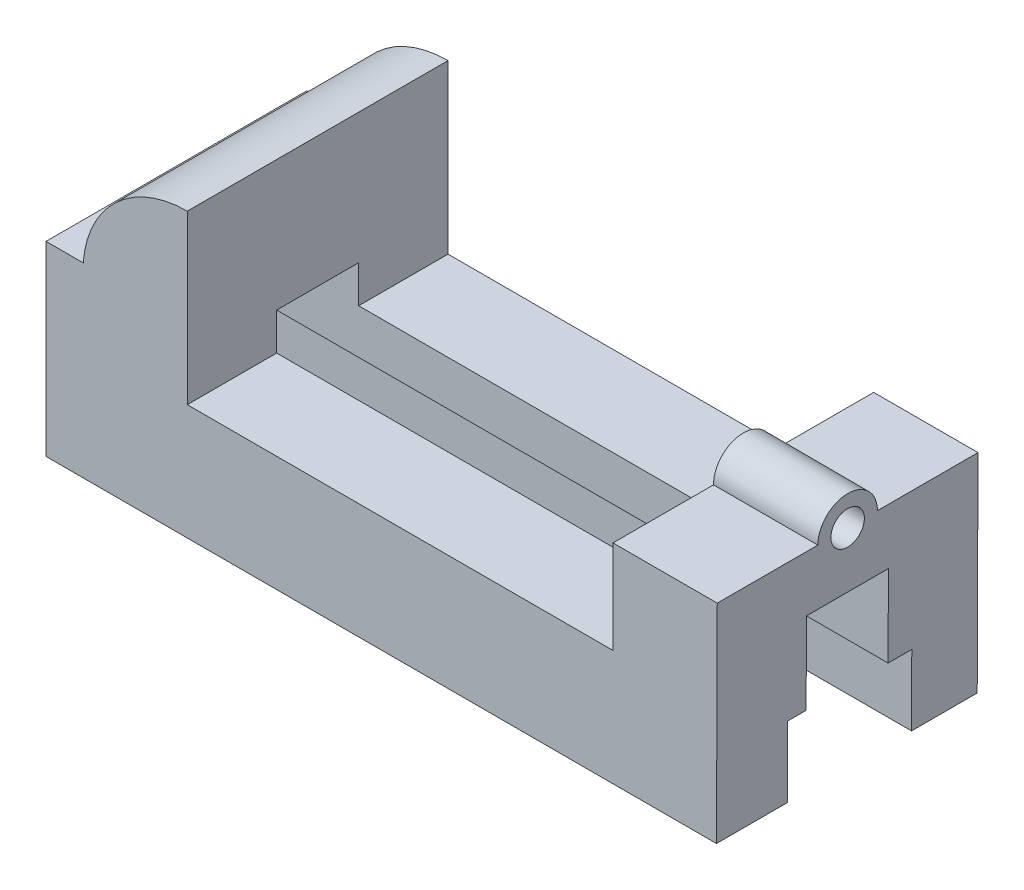
ISO-10303-21;
HEADER;
FILE_DESCRIPTION(('STEP AP214'),'2;1');
FILE_NAME('part.step','',(''),(''),'','','');
FILE_SCHEMA(('AUTOMOTIVE_DESIGN { 1 0 10303 214 1 1 1 1 }'));
ENDSEC;
DATA;
#1=APPLICATION_CONTEXT('core data for automotive mechanical design processes');
#2=APPLICATION_PROTOCOL_DEFINITION('international standard','automotive_design',2000,#1);
#3=PRODUCT_CONTEXT('',#1,'mechanical');
#4=PRODUCT('Part','Part','',(#3));
#5=PRODUCT_RELATED_PRODUCT_CATEGORY('part','',(#4));
#6=PRODUCT_DEFINITION_FORMATION('','',#4);
#7=PRODUCT_DEFINITION_CONTEXT('part definition',#1,'design');
#8=PRODUCT_DEFINITION('design','',#6,#7);
#9=PRODUCT_DEFINITION_SHAPE('','',#8);
#10=(LENGTH_UNIT() NAMED_UNIT(*) SI_UNIT(.MILLI.,.METRE.));
#11=(NAMED_UNIT(*) PLANE_ANGLE_UNIT() SI_UNIT($,.RADIAN.));
#12=(NAMED_UNIT(*) SI_UNIT($,.STERADIAN.) SOLID_ANGLE_UNIT());
#13=UNCERTAINTY_MEASURE_WITH_UNIT(LENGTH_MEASURE(1.E-05),#10,'distance_accuracy_value','');
#14=(GEOMETRIC_REPRESENTATION_CONTEXT(3) GLOBAL_UNCERTAINTY_ASSIGNED_CONTEXT((#13)) GLOBAL_UNIT_ASSIGNED_CONTEXT((#10,
#11,#12)) REPRESENTATION_CONTEXT('',''));
#15=CARTESIAN_POINT('',(0.,0.,0.));
#16=DIRECTION('',(0.,0.,1.));
#17=DIRECTION('',(1.,0.,0.));
#18=AXIS2_PLACEMENT_3D('',#15,#16,#17);
#19=CARTESIAN_POINT('',(152.209078325316,30.9996096973352,-70.));
#20=DIRECTION('',(0.,1.,0.));
#21=DIRECTION('',(-1.,0.,0.));
#22=AXIS2_PLACEMENT_3D('',#19,#20,#21);
#23=PLANE('',#22);
#24=DIRECTION('',(-1.,0.,0.));
#25=VECTOR('',#24,1.);
#26=CARTESIAN_POINT('',(152.209078325316,30.9996096973352,-46.));
#27=LINE('',#26,#25);
#28=CARTESIAN_POINT('',(152.209078325316,30.9996096973352,-46.));
#29=VERTEX_POINT('',#28);
#30=CARTESIAN_POINT('',(37.9284521346423,30.9996096973352,-46.));
#31=VERTEX_POINT('',#30);
#32=EDGE_CURVE('E288',#29,#31,#27,.T.);
#33=ORIENTED_EDGE('',*,*,#32,.F.);
#34=DIRECTION('',(0.,0.,1.));
#35=VECTOR('',#34,1.);
#36=CARTESIAN_POINT('',(152.209078325316,30.9996096973352,-70.));
#37=LINE('',#36,#35);
#38=CARTESIAN_POINT('',(152.209078325316,30.9996096973352,-70.));
#39=VERTEX_POINT('',#38);
#40=EDGE_CURVE('E364',#39,#29,#37,.T.);
#41=ORIENTED_EDGE('',*,*,#40,.F.);
#42=DIRECTION('',(-1.,0.,0.));
#43=VECTOR('',#42,1.);
#44=CARTESIAN_POINT('',(152.209078325316,30.9996096973352,-70.));
#45=LINE('',#44,#43);
#46=CARTESIAN_POINT('',(37.9284521346423,30.9996096973352,-70.));
#47=VERTEX_POINT('',#46);
#48=EDGE_CURVE('E324',#39,#47,#45,.T.);
#49=ORIENTED_EDGE('',*,*,#48,.T.);
#50=DIRECTION('',(0.,0.,1.));
#51=VECTOR('',#50,1.);
#52=CARTESIAN_POINT('',(37.9284521346423,30.9996096973352,-70.));
#53=LINE('',#52,#51);
#54=EDGE_CURVE('E363',#47,#31,#53,.T.);
#55=ORIENTED_EDGE('',*,*,#54,.T.);
#56=EDGE_LOOP('',(#33,#41,#49,#55));
#57=FACE_BOUND('',#56,.T.);
#58=ADVANCED_FACE('F39',(#57),#23,.T.);
#59=CARTESIAN_POINT('',(0.,0.,-70.));
#60=DIRECTION('',(0.,-1.,0.));
#61=DIRECTION('',(0.,0.,-1.));
#62=AXIS2_PLACEMENT_3D('',#59,#60,#61);
#63=PLANE('',#62);
#64=DIRECTION('',(1.,0.,0.));
#65=VECTOR('',#64,1.);
#66=CARTESIAN_POINT('',(0.,0.,-52.3591971480599));
#67=LINE('',#66,#65);
#68=CARTESIAN_POINT('',(0.,0.,-52.3591971480599));
#69=VERTEX_POINT('',#68);
#70=CARTESIAN_POINT('',(180.,0.,-52.3591971480599));
#71=VERTEX_POINT('',#70);
#72=EDGE_CURVE('E199',#69,#71,#67,.T.);
#73=ORIENTED_EDGE('',*,*,#72,.F.);
#74=DIRECTION('',(0.,0.,1.));
#75=VECTOR('',#74,1.);
#76=CARTESIAN_POINT('',(0.,0.,-70.));
#77=LINE('',#76,#75);
#78=CARTESIAN_POINT('',(0.,0.,-70.));
#79=VERTEX_POINT('',#78);
#80=EDGE_CURVE('E216',#79,#69,#77,.T.);
#81=ORIENTED_EDGE('',*,*,#80,.F.);
#82=DIRECTION('',(1.,0.,0.));
#83=VECTOR('',#82,1.);
#84=CARTESIAN_POINT('',(0.,0.,-70.));
#85=LINE('',#84,#83);
#86=CARTESIAN_POINT('',(180.,0.,-70.));
#87=VERTEX_POINT('',#86);
#88=EDGE_CURVE('E315',#79,#87,#85,.T.);
#89=ORIENTED_EDGE('',*,*,#88,.T.);
#90=DIRECTION('',(0.,0.,1.));
#91=VECTOR('',#90,1.);
#92=CARTESIAN_POINT('',(180.,0.,-70.));
#93=LINE('',#92,#91);
#94=EDGE_CURVE('E223',#87,#71,#93,.T.);
#95=ORIENTED_EDGE('',*,*,#94,.T.);
#96=EDGE_LOOP('',(#73,#81,#89,#95));
#97=FACE_BOUND('',#96,.T.);
#98=ADVANCED_FACE('F461',(#97),#63,.T.);
#99=CARTESIAN_POINT('',(180.209078325316,55.9996096973353,-70.));
#100=DIRECTION('',(0.,1.,0.));
#101=DIRECTION('',(0.,0.,1.));
#102=AXIS2_PLACEMENT_3D('',#99,#100,#101);
#103=PLANE('',#102);
#104=CARTESIAN_POINT('',(180.209078325316,55.9996096973353,-35.));
#105=DIRECTION('',(0.,1.,0.));
#106=DIRECTION('',(1.,0.,0.));
#107=AXIS2_PLACEMENT_3D('',#104,#105,#106);
#108=ELLIPSE('',#107,2142.73765261709,8.);
#109=CARTESIAN_POINT('',(180.209078325316,55.9996096973353,-43.));
#110=VERTEX_POINT('',#109);
#111=CARTESIAN_POINT('',(152.209078325316,55.9996096973353,-42.9993169435566));
#112=VERTEX_POINT('',#111);
#113=EDGE_CURVE('E307',#110,#112,#108,.T.);
#114=ORIENTED_EDGE('',*,*,#113,.F.);
#115=DIRECTION('',(0.,0.,1.));
#116=VECTOR('',#115,1.);
#117=CARTESIAN_POINT('',(180.209078325316,55.9996096973353,-70.));
#118=LINE('',#117,#116);
#119=CARTESIAN_POINT('',(180.209078325316,55.9996096973353,-70.));
#120=VERTEX_POINT('',#119);
#121=EDGE_CURVE('E375',#120,#110,#118,.T.);
#122=ORIENTED_EDGE('',*,*,#121,.F.);
#123=DIRECTION('',(-1.,0.,0.));
#124=VECTOR('',#123,1.);
#125=CARTESIAN_POINT('',(180.209078325316,55.9996096973353,-70.));
#126=LINE('',#125,#124);
#127=CARTESIAN_POINT('',(152.209078325316,55.9996096973353,-70.));
#128=VERTEX_POINT('',#127);
#129=EDGE_CURVE('E317',#120,#128,#126,.T.);
#130=ORIENTED_EDGE('',*,*,#129,.T.);
#131=DIRECTION('',(0.,0.,1.));
#132=VECTOR('',#131,1.);
#133=CARTESIAN_POINT('',(152.209078325316,55.9996096973353,-70.));
#134=LINE('',#133,#132);
#135=EDGE_CURVE('E369',#128,#112,#134,.T.);
#136=ORIENTED_EDGE('',*,*,#135,.T.);
#137=EDGE_LOOP('',(#114,#122,#130,#136));
#138=FACE_BOUND('',#137,.T.);
#139=ADVANCED_FACE('F413',(#138),#103,.T.);
#140=CARTESIAN_POINT('',(0.,50.,-70.));
#141=DIRECTION('',(-1.,0.,0.));
#142=DIRECTION('',(0.,-1.,0.));
#143=AXIS2_PLACEMENT_3D('',#140,#141,#142);
#144=PLANE('',#143);
#145=DIRECTION('',(0.,-1.,0.));
#146=VECTOR('',#145,1.);
#147=CARTESIAN_POINT('',(0.,0.,-52.3591971480599));
#148=LINE('',#147,#146);
#149=CARTESIAN_POINT('',(0.,19.,-52.3591971480599));
#150=VERTEX_POINT('',#149);
#151=EDGE_CURVE('E271',#150,#69,#148,.T.);
#152=ORIENTED_EDGE('',*,*,#151,.F.);
#153=DIRECTION('',(0.,0.,-1.));
#154=VECTOR('',#153,1.);
#155=CARTESIAN_POINT('',(0.,19.,-52.3591971480599));
#156=LINE('',#155,#154);
#157=CARTESIAN_POINT('',(0.,19.,-46.));
#158=VERTEX_POINT('',#157);
#159=EDGE_CURVE('E423',#158,#150,#156,.T.);
#160=ORIENTED_EDGE('',*,*,#159,.F.);
#161=DIRECTION('',(0.,-1.,0.));
#162=VECTOR('',#161,1.);
#163=CARTESIAN_POINT('',(0.,19.,-46.));
#164=LINE('',#163,#162);
#165=CARTESIAN_POINT('',(0.,41.,-46.));
#166=VERTEX_POINT('',#165);
#167=EDGE_CURVE('E652',#166,#158,#164,.T.);
#168=ORIENTED_EDGE('',*,*,#167,.F.);
#169=DIRECTION('',(0.,0.,-1.));
#170=VECTOR('',#169,1.);
#171=CARTESIAN_POINT('',(0.,41.,-46.));
#172=LINE('',#171,#170);
#173=CARTESIAN_POINT('',(0.,41.,-24.));
#174=VERTEX_POINT('',#173);
#175=EDGE_CURVE('E433',#174,#166,#172,.T.);
#176=ORIENTED_EDGE('',*,*,#175,.F.);
#177=DIRECTION('',(0.,1.,0.));
#178=VECTOR('',#177,1.);
#179=CARTESIAN_POINT('',(0.,41.,-24.));
#180=LINE('',#179,#178);
#181=CARTESIAN_POINT('',(0.,19.,-24.));
#182=VERTEX_POINT('',#181);
#183=EDGE_CURVE('E657',#182,#174,#180,.T.);
#184=ORIENTED_EDGE('',*,*,#183,.F.);
#185=DIRECTION('',(0.,0.,-1.));
#186=VECTOR('',#185,1.);
#187=CARTESIAN_POINT('',(0.,19.,-24.));
#188=LINE('',#187,#186);
#189=CARTESIAN_POINT('',(0.,19.,-19.));
#190=VERTEX_POINT('',#189);
#191=EDGE_CURVE('E209',#190,#182,#188,.T.);
#192=ORIENTED_EDGE('',*,*,#191,.F.);
#193=DIRECTION('',(0.,1.,0.));
#194=VECTOR('',#193,1.);
#195=CARTESIAN_POINT('',(0.,19.,-19.));
#196=LINE('',#195,#194);
#197=CARTESIAN_POINT('',(0.,0.,-19.));
#198=VERTEX_POINT('',#197);
#199=EDGE_CURVE('E191',#198,#190,#196,.T.);
#200=ORIENTED_EDGE('',*,*,#199,.F.);
#201=CARTESIAN_POINT('',(0.,0.,0.));
#202=VERTEX_POINT('',#201);
#203=EDGE_CURVE('E206',#198,#202,#77,.T.);
#204=ORIENTED_EDGE('',*,*,#203,.T.);
#205=DIRECTION('',(0.,-1.,0.));
#206=VECTOR('',#205,1.);
#207=CARTESIAN_POINT('',(0.,50.,0.));
#208=LINE('',#207,#206);
#209=CARTESIAN_POINT('',(0.,50.,0.));
#210=VERTEX_POINT('',#209);
#211=EDGE_CURVE('E334',#210,#202,#208,.T.);
#212=ORIENTED_EDGE('',*,*,#211,.F.);
#213=DIRECTION('',(0.,0.,1.));
#214=VECTOR('',#213,1.);
#215=CARTESIAN_POINT('',(0.,50.,-70.));
#216=LINE('',#215,#214);
#217=CARTESIAN_POINT('',(0.,50.,-70.));
#218=VERTEX_POINT('',#217);
#219=EDGE_CURVE('E203',#218,#210,#216,.T.);
#220=ORIENTED_EDGE('',*,*,#219,.F.);
#221=DIRECTION('',(0.,-1.,0.));
#222=VECTOR('',#221,1.);
#223=CARTESIAN_POINT('',(0.,50.,-70.));
#224=LINE('',#223,#222);
#225=EDGE_CURVE('E310',#218,#79,#224,.T.);
#226=ORIENTED_EDGE('',*,*,#225,.T.);
#227=ORIENTED_EDGE('',*,*,#80,.T.);
#228=EDGE_LOOP('',(#152,#160,#168,#176,#184,#192,#200,#204,#212,#220,#226,#227));
#229=FACE_BOUND('',#228,.T.);
#230=ADVANCED_FACE('F41',(#229),#144,.T.);
#231=CARTESIAN_POINT('',(10.,50.,-70.));
#232=DIRECTION('',(0.,1.,0.));
#233=DIRECTION('',(0.,0.,1.));
#234=AXIS2_PLACEMENT_3D('',#231,#232,#233);
#235=PLANE('',#234);
#236=DIRECTION('',(-1.,0.,0.));
#237=VECTOR('',#236,1.);
#238=CARTESIAN_POINT('',(10.,50.,0.));
#239=LINE('',#238,#237);
#240=CARTESIAN_POINT('',(10.,50.,0.));
#241=VERTEX_POINT('',#240);
#242=EDGE_CURVE('E311',#241,#210,#239,.T.);
#243=ORIENTED_EDGE('',*,*,#242,.F.);
#244=DIRECTION('',(0.,0.,1.));
#245=VECTOR('',#244,1.);
#246=CARTESIAN_POINT('',(10.,50.,-70.));
#247=LINE('',#246,#245);
#248=CARTESIAN_POINT('',(10.,50.,-70.));
#249=VERTEX_POINT('',#248);
#250=EDGE_CURVE('E360',#249,#241,#247,.T.);
#251=ORIENTED_EDGE('',*,*,#250,.F.);
#252=DIRECTION('',(-1.,0.,0.));
#253=VECTOR('',#252,1.);
#254=CARTESIAN_POINT('',(10.,50.,-70.));
#255=LINE('',#254,#253);
#256=EDGE_CURVE('E220',#249,#218,#255,.T.);
#257=ORIENTED_EDGE('',*,*,#256,.T.);
#258=ORIENTED_EDGE('',*,*,#219,.T.);
#259=EDGE_LOOP('',(#243,#251,#257,#258));
#260=FACE_BOUND('',#259,.T.);
#261=ADVANCED_FACE('F395',(#260),#235,.T.);
#262=CARTESIAN_POINT('',(37.9284521346423,47.9996096973352,-70.));
#263=DIRECTION('',(0.,0.,1.));
#264=DIRECTION('',(1.,0.,0.));
#265=AXIS2_PLACEMENT_3D('',#262,#263,#264);
#266=CYLINDRICAL_SURFACE('',#265,28.);
#267=CARTESIAN_POINT('',(37.9284521346423,47.9996096973352,0.));
#268=DIRECTION('',(0.,0.,1.));
#269=DIRECTION('',(1.,0.,0.));
#270=AXIS2_PLACEMENT_3D('',#267,#268,#269);
#271=CIRCLE('',#270,28.);
#272=CARTESIAN_POINT('',(37.9284521346423,75.9996096973352,0.));
#273=VERTEX_POINT('',#272);
#274=EDGE_CURVE('E351',#273,#241,#271,.T.);
#275=ORIENTED_EDGE('',*,*,#274,.F.);
#276=DIRECTION('',(0.,0.,1.));
#277=VECTOR('',#276,1.);
#278=CARTESIAN_POINT('',(37.9284521346423,75.9996096973352,-70.));
#279=LINE('',#278,#277);
#280=CARTESIAN_POINT('',(37.9284521346423,75.9996096973352,-70.));
#281=VERTEX_POINT('',#280);
#282=EDGE_CURVE('E359',#281,#273,#279,.T.);
#283=ORIENTED_EDGE('',*,*,#282,.F.);
#284=CARTESIAN_POINT('',(37.9284521346423,47.9996096973352,-70.));
#285=DIRECTION('',(0.,0.,1.));
#286=DIRECTION('',(1.,0.,0.));
#287=AXIS2_PLACEMENT_3D('',#284,#285,#286);
#288=CIRCLE('',#287,28.);
#289=EDGE_CURVE('E225',#281,#249,#288,.T.);
#290=ORIENTED_EDGE('',*,*,#289,.T.);
#291=ORIENTED_EDGE('',*,*,#250,.T.);
#292=EDGE_LOOP('',(#275,#283,#290,#291));
#293=FACE_BOUND('',#292,.T.);
#294=ADVANCED_FACE('F394',(#293),#266,.T.);
#295=CARTESIAN_POINT('',(37.9284521346423,30.9996096973352,-70.));
#296=DIRECTION('',(1.,0.,0.));
#297=DIRECTION('',(0.,0.,-1.));
#298=AXIS2_PLACEMENT_3D('',#295,#296,#297);
#299=PLANE('',#298);
#300=DIRECTION('',(0.,1.,0.));
#301=VECTOR('',#300,1.);
#302=CARTESIAN_POINT('',(37.9284521346423,30.9996096973352,-46.));
#303=LINE('',#302,#301);
#304=CARTESIAN_POINT('',(37.9284521346424,41.,-46.));
#305=VERTEX_POINT('',#304);
#306=EDGE_CURVE('E286',#31,#305,#303,.T.);
#307=ORIENTED_EDGE('',*,*,#306,.F.);
#308=ORIENTED_EDGE('',*,*,#54,.F.);
#309=DIRECTION('',(0.,1.,0.));
#310=VECTOR('',#309,1.);
#311=CARTESIAN_POINT('',(37.9284521346423,30.9996096973352,-70.));
#312=LINE('',#311,#310);
#313=EDGE_CURVE('E327',#47,#281,#312,.T.);
#314=ORIENTED_EDGE('',*,*,#313,.T.);
#315=ORIENTED_EDGE('',*,*,#282,.T.);
#316=DIRECTION('',(0.,1.,0.));
#317=VECTOR('',#316,1.);
#318=CARTESIAN_POINT('',(37.9284521346423,30.9996096973352,0.));
#319=LINE('',#318,#317);
#320=CARTESIAN_POINT('',(37.9284521346423,30.9996096973352,0.));
#321=VERTEX_POINT('',#320);
#322=EDGE_CURVE('E346',#321,#273,#319,.T.);
#323=ORIENTED_EDGE('',*,*,#322,.F.);
#324=CARTESIAN_POINT('',(37.9284521346423,30.9996096973352,-24.));
#325=VERTEX_POINT('',#324);
#326=EDGE_CURVE('E365',#325,#321,#53,.T.);
#327=ORIENTED_EDGE('',*,*,#326,.F.);
#328=DIRECTION('',(0.,-1.,0.));
#329=VECTOR('',#328,1.);
#330=CARTESIAN_POINT('',(37.9284521346423,30.9996096973352,-24.));
#331=LINE('',#330,#329);
#332=CARTESIAN_POINT('',(37.9284521346424,41.,-24.));
#333=VERTEX_POINT('',#332);
#334=EDGE_CURVE('E281',#333,#325,#331,.T.);
#335=ORIENTED_EDGE('',*,*,#334,.F.);
#336=DIRECTION('',(0.,0.,1.));
#337=VECTOR('',#336,1.);
#338=CARTESIAN_POINT('',(37.9284521346423,41.,-70.));
#339=LINE('',#338,#337);
#340=EDGE_CURVE('E283',#305,#333,#339,.T.);
#341=ORIENTED_EDGE('',*,*,#340,.F.);
#342=EDGE_LOOP('',(#307,#308,#314,#315,#323,#327,#335,#341));
#343=FACE_BOUND('',#342,.T.);
#344=ADVANCED_FACE('F396',(#343),#299,.T.);
#345=DIRECTION('',(1.,0.,0.));
#346=VECTOR('',#345,1.);
#347=CARTESIAN_POINT('',(152.209078325316,30.9996096973352,-24.));
#348=LINE('',#347,#346);
#349=CARTESIAN_POINT('',(152.209078325316,30.9996096973352,-24.));
#350=VERTEX_POINT('',#349);
#351=EDGE_CURVE('E53',#325,#350,#348,.T.);
#352=ORIENTED_EDGE('',*,*,#351,.F.);
#353=ORIENTED_EDGE('',*,*,#326,.T.);
#354=DIRECTION('',(-1.,0.,0.));
#355=VECTOR('',#354,1.);
#356=CARTESIAN_POINT('',(152.209078325316,30.9996096973352,0.));
#357=LINE('',#356,#355);
#358=CARTESIAN_POINT('',(152.209078325316,30.9996096973352,0.));
#359=VERTEX_POINT('',#358);
#360=EDGE_CURVE('E341',#359,#321,#357,.T.);
#361=ORIENTED_EDGE('',*,*,#360,.F.);
#362=EDGE_CURVE('E366',#350,#359,#37,.T.);
#363=ORIENTED_EDGE('',*,*,#362,.F.);
#364=EDGE_LOOP('',(#352,#353,#361,#363));
#365=FACE_BOUND('',#364,.T.);
#366=ADVANCED_FACE('F437',(#365),#23,.T.);
#367=CARTESIAN_POINT('',(152.209078325316,55.9996096973353,-70.));
#368=DIRECTION('',(-1.,0.,0.));
#369=DIRECTION('',(0.,0.,1.));
#370=AXIS2_PLACEMENT_3D('',#367,#368,#369);
#371=PLANE('',#370);
#372=DIRECTION('',(0.,-1.,0.));
#373=VECTOR('',#372,1.);
#374=CARTESIAN_POINT('',(152.209078325316,55.9996096973353,-46.));
#375=LINE('',#374,#373);
#376=CARTESIAN_POINT('',(152.209078325316,41.,-46.));
#377=VERTEX_POINT('',#376);
#378=EDGE_CURVE('E287',#377,#29,#375,.T.);
#379=ORIENTED_EDGE('',*,*,#378,.F.);
#380=DIRECTION('',(0.,0.,-1.));
#381=VECTOR('',#380,1.);
#382=CARTESIAN_POINT('',(152.209078325316,41.,-70.));
#383=LINE('',#382,#381);
#384=CARTESIAN_POINT('',(152.209078325316,41.,-24.));
#385=VERTEX_POINT('',#384);
#386=EDGE_CURVE('E252',#385,#377,#383,.T.);
#387=ORIENTED_EDGE('',*,*,#386,.F.);
#388=DIRECTION('',(0.,1.,0.));
#389=VECTOR('',#388,1.);
#390=CARTESIAN_POINT('',(152.209078325316,55.9996096973353,-24.));
#391=LINE('',#390,#389);
#392=EDGE_CURVE('E279',#350,#385,#391,.T.);
#393=ORIENTED_EDGE('',*,*,#392,.F.);
#394=ORIENTED_EDGE('',*,*,#362,.T.);
#395=DIRECTION('',(0.,-1.,0.));
#396=VECTOR('',#395,1.);
#397=CARTESIAN_POINT('',(152.209078325316,55.9996096973353,0.));
#398=LINE('',#397,#396);
#399=CARTESIAN_POINT('',(152.209078325316,55.9996096973353,0.));
#400=VERTEX_POINT('',#399);
#401=EDGE_CURVE('E345',#400,#359,#398,.T.);
#402=ORIENTED_EDGE('',*,*,#401,.F.);
#403=CARTESIAN_POINT('',(152.209078325316,55.9996096973353,-27.0006830564435));
#404=VERTEX_POINT('',#403);
#405=EDGE_CURVE('E371',#404,#400,#134,.T.);
#406=ORIENTED_EDGE('',*,*,#405,.F.);
#407=CARTESIAN_POINT('',(152.209078325316,56.1041495886038,-35.));
#408=DIRECTION('',(-1.,0.,0.));
#409=DIRECTION('',(0.,-1.,0.));
#410=AXIS2_PLACEMENT_3D('',#407,#408,#409);
#411=ELLIPSE('',#410,8.00005575791215,8.);
#412=EDGE_CURVE('E308',#112,#404,#411,.T.);
#413=ORIENTED_EDGE('',*,*,#412,.F.);
#414=ORIENTED_EDGE('',*,*,#135,.F.);
#415=DIRECTION('',(0.,-1.,0.));
#416=VECTOR('',#415,1.);
#417=CARTESIAN_POINT('',(152.209078325316,55.9996096973353,-70.));
#418=LINE('',#417,#416);
#419=EDGE_CURVE('E325',#128,#39,#418,.T.);
#420=ORIENTED_EDGE('',*,*,#419,.T.);
#421=ORIENTED_EDGE('',*,*,#40,.T.);
#422=EDGE_LOOP('',(#379,#387,#393,#394,#402,#406,#413,#414,#420,#421));
#423=FACE_BOUND('',#422,.T.);
#424=ADVANCED_FACE('F407',(#423),#371,.T.);
#425=CARTESIAN_POINT('',(180.209078325316,55.9996096973353,-27.));
#426=VERTEX_POINT('',#425);
#427=EDGE_CURVE('E305',#404,#426,#108,.T.);
#428=ORIENTED_EDGE('',*,*,#427,.F.);
#429=ORIENTED_EDGE('',*,*,#405,.T.);
#430=DIRECTION('',(-1.,0.,0.));
#431=VECTOR('',#430,1.);
#432=CARTESIAN_POINT('',(180.209078325316,55.9996096973353,0.));
#433=LINE('',#432,#431);
#434=CARTESIAN_POINT('',(180.209078325316,55.9996096973353,0.));
#435=VERTEX_POINT('',#434);
#436=EDGE_CURVE('E338',#435,#400,#433,.T.);
#437=ORIENTED_EDGE('',*,*,#436,.F.);
#438=EDGE_CURVE('E372',#426,#435,#118,.T.);
#439=ORIENTED_EDGE('',*,*,#438,.F.);
#440=EDGE_LOOP('',(#428,#429,#437,#439));
#441=FACE_BOUND('',#440,.T.);
#442=ADVANCED_FACE('F444',(#441),#103,.T.);
#443=CARTESIAN_POINT('',(180.,0.,-70.));
#444=DIRECTION('',(0.999993030309558,-0.00373354152349401,0.));
#445=DIRECTION('',(0.00373354152349401,0.999993030309558,0.));
#446=AXIS2_PLACEMENT_3D('',#443,#444,#445);
#447=PLANE('',#446);
#448=DIRECTION('',(0.00373354152349401,0.999993030309558,0.));
#449=VECTOR('',#448,1.);
#450=CARTESIAN_POINT('',(180.,0.,-52.3591971480599));
#451=LINE('',#450,#449);
#452=CARTESIAN_POINT('',(180.070937783361,19.,-52.3591971480599));
#453=VERTEX_POINT('',#452);
#454=EDGE_CURVE('E274',#71,#453,#451,.T.);
#455=ORIENTED_EDGE('',*,*,#454,.F.);
#456=ORIENTED_EDGE('',*,*,#94,.F.);
#457=DIRECTION('',(0.00373354152349401,0.999993030309558,0.));
#458=VECTOR('',#457,1.);
#459=CARTESIAN_POINT('',(180.,0.,-70.));
#460=LINE('',#459,#458);
#461=EDGE_CURVE('E316',#87,#120,#460,.T.);
#462=ORIENTED_EDGE('',*,*,#461,.T.);
#463=ORIENTED_EDGE('',*,*,#121,.T.);
#464=CARTESIAN_POINT('',(180.209078325316,55.9996096973353,-35.));
#465=DIRECTION('',(0.999993030309558,-0.00373354152349401,0.));
#466=DIRECTION('',(0.00373354152349401,0.999993030309558,0.));
#467=AXIS2_PLACEMENT_3D('',#464,#465,#466);
#468=CIRCLE('',#467,8.);
#469=EDGE_CURVE('E296',#110,#426,#468,.T.);
#470=ORIENTED_EDGE('',*,*,#469,.T.);
#471=ORIENTED_EDGE('',*,*,#438,.T.);
#472=DIRECTION('',(0.00373354152349401,0.999993030309558,0.));
#473=VECTOR('',#472,1.);
#474=CARTESIAN_POINT('',(180.,0.,0.));
#475=LINE('',#474,#473);
#476=CARTESIAN_POINT('',(180.,0.,0.));
#477=VERTEX_POINT('',#476);
#478=EDGE_CURVE('E336',#477,#435,#475,.T.);
#479=ORIENTED_EDGE('',*,*,#478,.F.);
#480=CARTESIAN_POINT('',(180.,0.,-19.));
#481=VERTEX_POINT('',#480);
#482=EDGE_CURVE('E219',#481,#477,#93,.T.);
#483=ORIENTED_EDGE('',*,*,#482,.F.);
#484=DIRECTION('',(-0.00373354152349401,-0.999993030309558,0.));
#485=VECTOR('',#484,1.);
#486=CARTESIAN_POINT('',(180.,0.,-19.));
#487=LINE('',#486,#485);
#488=CARTESIAN_POINT('',(180.070937783361,19.,-19.));
#489=VERTEX_POINT('',#488);
#490=EDGE_CURVE('E65',#489,#481,#487,.T.);
#491=ORIENTED_EDGE('',*,*,#490,.F.);
#492=DIRECTION('',(0.,0.,1.));
#493=VECTOR('',#492,1.);
#494=CARTESIAN_POINT('',(180.070937783361,19.,-70.));
#495=LINE('',#494,#493);
#496=CARTESIAN_POINT('',(180.070937783361,19.,-24.));
#497=VERTEX_POINT('',#496);
#498=EDGE_CURVE('E228',#497,#489,#495,.T.);
#499=ORIENTED_EDGE('',*,*,#498,.F.);
#500=DIRECTION('',(-0.00373354152349401,-0.999993030309558,0.));
#501=VECTOR('',#500,1.);
#502=CARTESIAN_POINT('',(180.,0.,-24.));
#503=LINE('',#502,#501);
#504=CARTESIAN_POINT('',(180.153076269357,41.,-24.));
#505=VERTEX_POINT('',#504);
#506=EDGE_CURVE('E232',#505,#497,#503,.T.);
#507=ORIENTED_EDGE('',*,*,#506,.F.);
#508=DIRECTION('',(0.,0.,1.));
#509=VECTOR('',#508,1.);
#510=CARTESIAN_POINT('',(180.153076269357,41.,-70.));
#511=LINE('',#510,#509);
#512=CARTESIAN_POINT('',(180.153076269357,41.,-46.));
#513=VERTEX_POINT('',#512);
#514=EDGE_CURVE('E233',#513,#505,#511,.T.);
#515=ORIENTED_EDGE('',*,*,#514,.F.);
#516=DIRECTION('',(0.00373354152349401,0.999993030309558,0.));
#517=VECTOR('',#516,1.);
#518=CARTESIAN_POINT('',(180.,0.,-46.));
#519=LINE('',#518,#517);
#520=CARTESIAN_POINT('',(180.070937783361,19.,-46.));
#521=VERTEX_POINT('',#520);
#522=EDGE_CURVE('E50',#521,#513,#519,.T.);
#523=ORIENTED_EDGE('',*,*,#522,.F.);
#524=DIRECTION('',(0.,0.,1.));
#525=VECTOR('',#524,1.);
#526=CARTESIAN_POINT('',(180.070937783361,19.,-70.));
#527=LINE('',#526,#525);
#528=EDGE_CURVE('E11',#453,#521,#527,.T.);
#529=ORIENTED_EDGE('',*,*,#528,.F.);
#530=EDGE_LOOP('',(#455,#456,#462,#463,#470,#471,#479,#483,#491,#499,#507,#515,#523,#529));
#531=FACE_BOUND('',#530,.T.);
#532=CARTESIAN_POINT('',(180.209078325316,55.9996096973353,-35.));
#533=DIRECTION('',(0.999993030309558,-0.00373354152349401,0.));
#534=DIRECTION('',(0.00373354152349401,0.999993030309558,0.));
#535=AXIS2_PLACEMENT_3D('',#532,#533,#534);
#536=CIRCLE('',#535,4.5);
#537=CARTESIAN_POINT('',(180.225879262171,60.4995783337283,-35.));
#538=VERTEX_POINT('',#537);
#539=EDGE_CURVE('E295',#538,#538,#536,.T.);
#540=ORIENTED_EDGE('',*,*,#539,.F.);
#541=EDGE_LOOP('',(#540));
#542=FACE_BOUND('',#541,.T.);
#543=ADVANCED_FACE('F260',(#531,#542),#447,.T.);
#544=DIRECTION('',(-1.,0.,0.));
#545=VECTOR('',#544,1.);
#546=CARTESIAN_POINT('',(0.,0.,-19.));
#547=LINE('',#546,#545);
#548=EDGE_CURVE('E195',#481,#198,#547,.T.);
#549=ORIENTED_EDGE('',*,*,#548,.F.);
#550=ORIENTED_EDGE('',*,*,#482,.T.);
#551=DIRECTION('',(1.,0.,0.));
#552=VECTOR('',#551,1.);
#553=CARTESIAN_POINT('',(0.,0.,0.));
#554=LINE('',#553,#552);
#555=EDGE_CURVE('E212',#202,#477,#554,.T.);
#556=ORIENTED_EDGE('',*,*,#555,.F.);
#557=ORIENTED_EDGE('',*,*,#203,.F.);
#558=EDGE_LOOP('',(#549,#550,#556,#557));
#559=FACE_BOUND('',#558,.T.);
#560=ADVANCED_FACE('F215',(#559),#63,.T.);
#561=CARTESIAN_POINT('',(37.9284521346423,47.9996096973352,-70.));
#562=DIRECTION('',(0.,0.,1.));
#563=DIRECTION('',(1.,0.,0.));
#564=AXIS2_PLACEMENT_3D('',#561,#562,#563);
#565=PLANE('',#564);
#566=ORIENTED_EDGE('',*,*,#225,.F.);
#567=ORIENTED_EDGE('',*,*,#256,.F.);
#568=ORIENTED_EDGE('',*,*,#289,.F.);
#569=ORIENTED_EDGE('',*,*,#313,.F.);
#570=ORIENTED_EDGE('',*,*,#48,.F.);
#571=ORIENTED_EDGE('',*,*,#419,.F.);
#572=ORIENTED_EDGE('',*,*,#129,.F.);
#573=ORIENTED_EDGE('',*,*,#461,.F.);
#574=ORIENTED_EDGE('',*,*,#88,.F.);
#575=EDGE_LOOP('',(#566,#567,#568,#569,#570,#571,#572,#573,#574));
#576=FACE_BOUND('',#575,.T.);
#577=ADVANCED_FACE('F386',(#576),#565,.F.);
#578=CARTESIAN_POINT('',(37.9284521346423,47.9996096973352,0.));
#579=DIRECTION('',(0.,0.,1.));
#580=DIRECTION('',(1.,0.,0.));
#581=AXIS2_PLACEMENT_3D('',#578,#579,#580);
#582=PLANE('',#581);
#583=ORIENTED_EDGE('',*,*,#211,.T.);
#584=ORIENTED_EDGE('',*,*,#555,.T.);
#585=ORIENTED_EDGE('',*,*,#478,.T.);
#586=ORIENTED_EDGE('',*,*,#436,.T.);
#587=ORIENTED_EDGE('',*,*,#401,.T.);
#588=ORIENTED_EDGE('',*,*,#360,.T.);
#589=ORIENTED_EDGE('',*,*,#322,.T.);
#590=ORIENTED_EDGE('',*,*,#274,.T.);
#591=ORIENTED_EDGE('',*,*,#242,.T.);
#592=EDGE_LOOP('',(#583,#584,#585,#586,#587,#588,#589,#590,#591));
#593=FACE_BOUND('',#592,.T.);
#594=ADVANCED_FACE('F385',(#593),#582,.T.);
#595=CARTESIAN_POINT('',(152.209273476648,56.1041488599931,-35.));
#596=DIRECTION('',(0.999993030309558,-0.00373354152349401,0.));
#597=DIRECTION('',(0.00373354152349401,0.999993030309558,0.));
#598=AXIS2_PLACEMENT_3D('',#595,#596,#597);
#599=CYLINDRICAL_SURFACE('',#598,8.);
#600=CARTESIAN_POINT('',(152.209273476648,56.1041488599931,-35.));
#601=DIRECTION('',(0.999993030309558,-0.00373354152349401,0.));
#602=DIRECTION('',(0.00373354152349401,0.999993030309558,0.));
#603=AXIS2_PLACEMENT_3D('',#600,#601,#602);
#604=CIRCLE('',#603,8.);
#605=CARTESIAN_POINT('',(152.239141808836,64.1040931024695,-35.));
#606=VERTEX_POINT('',#605);
#607=EDGE_CURVE('E298',#606,#606,#604,.T.);
#608=ORIENTED_EDGE('',*,*,#607,.T.);
#609=EDGE_LOOP('',(#608));
#610=FACE_BOUND('',#609,.T.);
#611=ORIENTED_EDGE('',*,*,#469,.F.);
#612=ORIENTED_EDGE('',*,*,#113,.T.);
#613=ORIENTED_EDGE('',*,*,#412,.T.);
#614=ORIENTED_EDGE('',*,*,#427,.T.);
#615=EDGE_LOOP('',(#611,#612,#613,#614));
#616=FACE_BOUND('',#615,.T.);
#617=ADVANCED_FACE('F443',(#610,#616),#599,.T.);
#618=CARTESIAN_POINT('',(152.209273476648,56.1041488599931,-35.));
#619=DIRECTION('',(0.999993030309558,-0.00373354152349401,0.));
#620=DIRECTION('',(0.00373354152349401,0.999993030309558,0.));
#621=AXIS2_PLACEMENT_3D('',#618,#619,#620);
#622=PLANE('',#621);
#623=CARTESIAN_POINT('',(152.209273476648,56.1041488599931,-35.));
#624=DIRECTION('',(0.999993030309558,-0.00373354152349401,0.));
#625=DIRECTION('',(0.00373354152349401,0.999993030309558,0.));
#626=AXIS2_PLACEMENT_3D('',#623,#624,#625);
#627=CIRCLE('',#626,4.5);
#628=CARTESIAN_POINT('',(152.226074413504,60.6041174963861,-35.));
#629=VERTEX_POINT('',#628);
#630=EDGE_CURVE('E291',#629,#629,#627,.T.);
#631=ORIENTED_EDGE('',*,*,#630,.T.);
#632=EDGE_LOOP('',(#631));
#633=FACE_BOUND('',#632,.T.);
#634=ORIENTED_EDGE('',*,*,#607,.F.);
#635=EDGE_LOOP('',(#634));
#636=FACE_BOUND('',#635,.T.);
#637=ADVANCED_FACE('F450',(#633,#636),#622,.F.);
#638=CARTESIAN_POINT('',(152.209273476648,56.1041488599931,-35.));
#639=DIRECTION('',(0.999993030309558,-0.00373354152349401,0.));
#640=DIRECTION('',(0.00373354152349401,0.999993030309558,0.));
#641=AXIS2_PLACEMENT_3D('',#638,#639,#640);
#642=CYLINDRICAL_SURFACE('',#641,4.5);
#643=ORIENTED_EDGE('',*,*,#630,.F.);
#644=EDGE_LOOP('',(#643));
#645=FACE_BOUND('',#644,.T.);
#646=ORIENTED_EDGE('',*,*,#539,.T.);
#647=EDGE_LOOP('',(#646));
#648=FACE_BOUND('',#647,.T.);
#649=ADVANCED_FACE('F454',(#645,#648),#642,.F.);
#650=CARTESIAN_POINT('',(180.238946657504,41.,-46.));
#651=DIRECTION('',(0.,1.,0.));
#652=DIRECTION('',(-1.,0.,0.));
#653=AXIS2_PLACEMENT_3D('',#650,#651,#652);
#654=PLANE('',#653);
#655=ORIENTED_EDGE('',*,*,#340,.T.);
#656=DIRECTION('',(-1.,0.,0.));
#657=VECTOR('',#656,1.);
#658=CARTESIAN_POINT('',(180.238946657504,41.,-24.));
#659=LINE('',#658,#657);
#660=EDGE_CURVE('E270',#333,#174,#659,.T.);
#661=ORIENTED_EDGE('',*,*,#660,.T.);
#662=ORIENTED_EDGE('',*,*,#175,.T.);
#663=DIRECTION('',(-1.,0.,0.));
#664=VECTOR('',#663,1.);
#665=CARTESIAN_POINT('',(180.238946657504,41.,-46.));
#666=LINE('',#665,#664);
#667=EDGE_CURVE('E251',#305,#166,#666,.T.);
#668=ORIENTED_EDGE('',*,*,#667,.F.);
#669=EDGE_LOOP('',(#655,#661,#662,#668));
#670=FACE_BOUND('',#669,.T.);
#671=ADVANCED_FACE('F429',(#670),#654,.F.);
#672=CARTESIAN_POINT('',(180.238946657504,0.,-52.3591971480599));
#673=DIRECTION('',(0.,0.,-1.));
#674=DIRECTION('',(-1.,0.,0.));
#675=AXIS2_PLACEMENT_3D('',#672,#673,#674);
#676=PLANE('',#675);
#677=ORIENTED_EDGE('',*,*,#454,.T.);
#678=DIRECTION('',(-1.,0.,0.));
#679=VECTOR('',#678,1.);
#680=CARTESIAN_POINT('',(180.238946657504,19.,-52.3591971480599));
#681=LINE('',#680,#679);
#682=EDGE_CURVE('E277',#453,#150,#681,.T.);
#683=ORIENTED_EDGE('',*,*,#682,.T.);
#684=ORIENTED_EDGE('',*,*,#151,.T.);
#685=ORIENTED_EDGE('',*,*,#72,.T.);
#686=EDGE_LOOP('',(#677,#683,#684,#685));
#687=FACE_BOUND('',#686,.T.);
#688=ADVANCED_FACE('F418',(#687),#676,.F.);
#689=CARTESIAN_POINT('',(180.238946657504,19.,-52.3591971480599));
#690=DIRECTION('',(0.,1.,0.));
#691=DIRECTION('',(-1.,0.,0.));
#692=AXIS2_PLACEMENT_3D('',#689,#690,#691);
#693=PLANE('',#692);
#694=ORIENTED_EDGE('',*,*,#528,.T.);
#695=DIRECTION('',(-1.,0.,0.));
#696=VECTOR('',#695,1.);
#697=CARTESIAN_POINT('',(180.238946657504,19.,-46.));
#698=LINE('',#697,#696);
#699=EDGE_CURVE('E242',#521,#158,#698,.T.);
#700=ORIENTED_EDGE('',*,*,#699,.T.);
#701=ORIENTED_EDGE('',*,*,#159,.T.);
#702=ORIENTED_EDGE('',*,*,#682,.F.);
#703=EDGE_LOOP('',(#694,#700,#701,#702));
#704=FACE_BOUND('',#703,.T.);
#705=ADVANCED_FACE('F420',(#704),#693,.F.);
#706=CARTESIAN_POINT('',(180.238946657504,19.,-46.));
#707=DIRECTION('',(0.,0.,-1.));
#708=DIRECTION('',(-1.,0.,0.));
#709=AXIS2_PLACEMENT_3D('',#706,#707,#708);
#710=PLANE('',#709);
#711=ORIENTED_EDGE('',*,*,#306,.T.);
#712=ORIENTED_EDGE('',*,*,#667,.T.);
#713=ORIENTED_EDGE('',*,*,#167,.T.);
#714=ORIENTED_EDGE('',*,*,#699,.F.);
#715=ORIENTED_EDGE('',*,*,#522,.T.);
#716=EDGE_CURVE('E238',#513,#377,#666,.T.);
#717=ORIENTED_EDGE('',*,*,#716,.T.);
#718=ORIENTED_EDGE('',*,*,#378,.T.);
#719=ORIENTED_EDGE('',*,*,#32,.T.);
#720=EDGE_LOOP('',(#711,#712,#713,#714,#715,#717,#718,#719));
#721=FACE_BOUND('',#720,.T.);
#722=ADVANCED_FACE('F239',(#721),#710,.F.);
#723=ORIENTED_EDGE('',*,*,#386,.T.);
#724=ORIENTED_EDGE('',*,*,#716,.F.);
#725=ORIENTED_EDGE('',*,*,#514,.T.);
#726=EDGE_CURVE('E262',#505,#385,#659,.T.);
#727=ORIENTED_EDGE('',*,*,#726,.T.);
#728=EDGE_LOOP('',(#723,#724,#725,#727));
#729=FACE_BOUND('',#728,.T.);
#730=ADVANCED_FACE('F248',(#729),#654,.F.);
#731=CARTESIAN_POINT('',(180.238946657504,41.,-24.));
#732=DIRECTION('',(0.,0.,1.));
#733=DIRECTION('',(0.,-1.,0.));
#734=AXIS2_PLACEMENT_3D('',#731,#732,#733);
#735=PLANE('',#734);
#736=ORIENTED_EDGE('',*,*,#334,.T.);
#737=ORIENTED_EDGE('',*,*,#351,.T.);
#738=ORIENTED_EDGE('',*,*,#392,.T.);
#739=ORIENTED_EDGE('',*,*,#726,.F.);
#740=ORIENTED_EDGE('',*,*,#506,.T.);
#741=DIRECTION('',(-1.,0.,0.));
#742=VECTOR('',#741,1.);
#743=CARTESIAN_POINT('',(180.238946657504,19.,-24.));
#744=LINE('',#743,#742);
#745=EDGE_CURVE('E263',#497,#182,#744,.T.);
#746=ORIENTED_EDGE('',*,*,#745,.T.);
#747=ORIENTED_EDGE('',*,*,#183,.T.);
#748=ORIENTED_EDGE('',*,*,#660,.F.);
#749=EDGE_LOOP('',(#736,#737,#738,#739,#740,#746,#747,#748));
#750=FACE_BOUND('',#749,.T.);
#751=ADVANCED_FACE('F261',(#750),#735,.F.);
#752=CARTESIAN_POINT('',(180.238946657504,19.,-24.));
#753=DIRECTION('',(0.,1.,0.));
#754=DIRECTION('',(-1.,0.,0.));
#755=AXIS2_PLACEMENT_3D('',#752,#753,#754);
#756=PLANE('',#755);
#757=ORIENTED_EDGE('',*,*,#498,.T.);
#758=DIRECTION('',(-1.,0.,0.));
#759=VECTOR('',#758,1.);
#760=CARTESIAN_POINT('',(180.238946657504,19.,-19.));
#761=LINE('',#760,#759);
#762=EDGE_CURVE('E268',#489,#190,#761,.T.);
#763=ORIENTED_EDGE('',*,*,#762,.T.);
#764=ORIENTED_EDGE('',*,*,#191,.T.);
#765=ORIENTED_EDGE('',*,*,#745,.F.);
#766=EDGE_LOOP('',(#757,#763,#764,#765));
#767=FACE_BOUND('',#766,.T.);
#768=ADVANCED_FACE('F266',(#767),#756,.F.);
#769=CARTESIAN_POINT('',(180.238946657504,19.,-19.));
#770=DIRECTION('',(0.,0.,1.));
#771=DIRECTION('',(0.,-1.,0.));
#772=AXIS2_PLACEMENT_3D('',#769,#770,#771);
#773=PLANE('',#772);
#774=ORIENTED_EDGE('',*,*,#490,.T.);
#775=ORIENTED_EDGE('',*,*,#548,.T.);
#776=ORIENTED_EDGE('',*,*,#199,.T.);
#777=ORIENTED_EDGE('',*,*,#762,.F.);
#778=EDGE_LOOP('',(#774,#775,#776,#777));
#779=FACE_BOUND('',#778,.T.);
#780=ADVANCED_FACE('F194',(#779),#773,.F.);
#781=CLOSED_SHELL('',(#58,#98,#139,#230,#261,#294,#344,#366,#424,#442,#543,#560,#577,#594,#617,
#637,#649,#671,#688,#705,#722,#730,#751,#768,#780));
#782=MANIFOLD_SOLID_BREP('B2',#781);
#783=ADVANCED_BREP_SHAPE_REPRESENTATION('',(#18,#782),#14);
#784=SHAPE_DEFINITION_REPRESENTATION(#9,#783);
ENDSEC;
END-ISO-10303-21;
